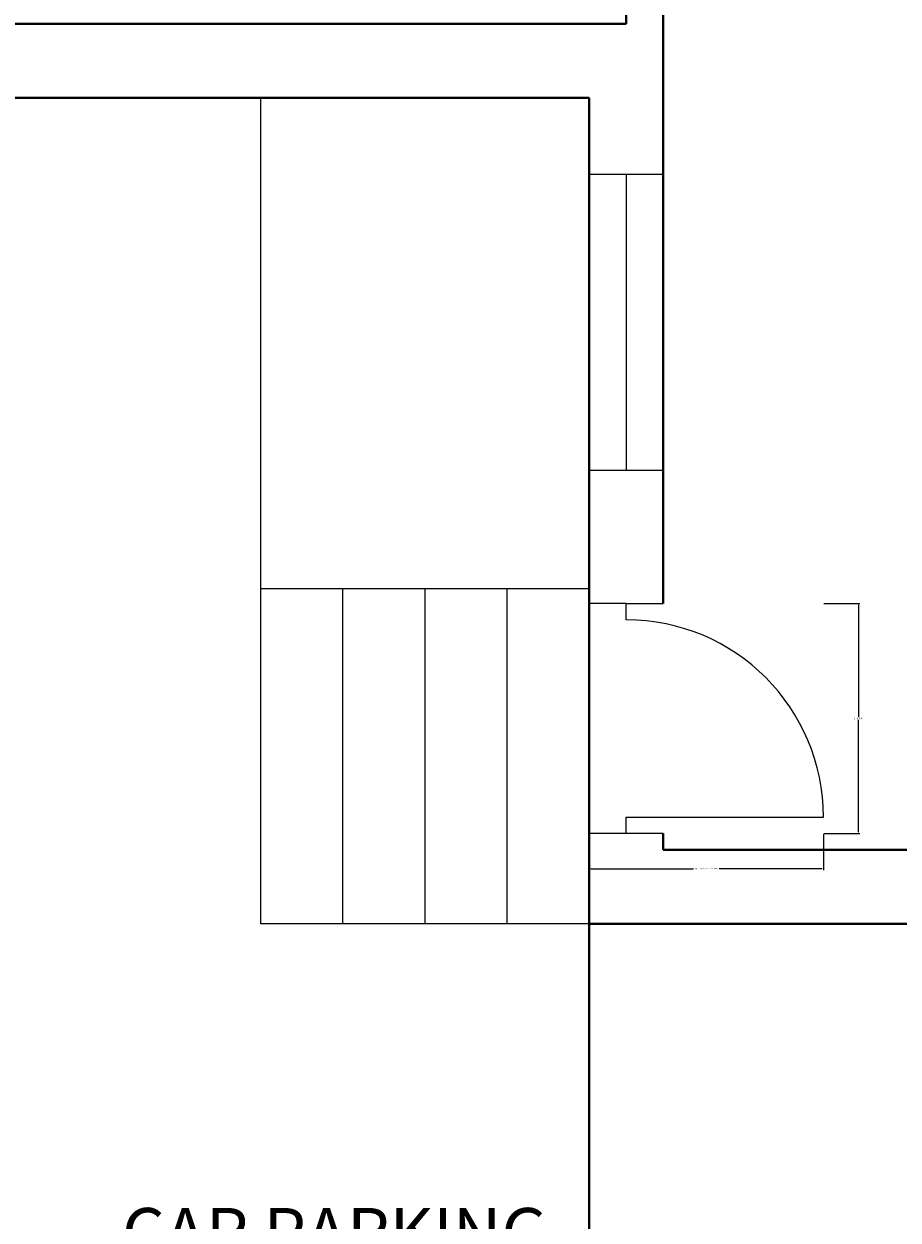
# Model space of a CAD drawing. Units: inches. Extents: x -19 to 419, y -828 to 43.
# Tile 4 of 9: x 126 to 233, y -720 to -574. Entities that reach past the tile are written whole.
import ezdxf

# ---------------------------------------------------------------- set-up
doc = ezdxf.new("R2010")
doc.units = ezdxf.units.IN
doc.header["$MEASUREMENT"] = 0
for name, color, linetype, lineweight in [('A-ANNO-DIMS', 2, 'Continuous', 18), ('A-AREA-IDEN', 7, 'Continuous', 25), ('A-DOOR', 3, 'Continuous', 25), ('A-FLOR-STRS', 7, 'Continuous', 25), ('A-GLAZ', 4, 'Continuous', 20), ('A-WALL', 7, 'Continuous', 40)]:
    doc.layers.add(name, color=color, linetype=linetype, lineweight=lineweight)
doc.styles.get("Standard").update_dxf_attribs({"font": 'arial.ttf'})
doc.dimstyles.get("Standard").update_dxf_attribs({"dimtxt": 0.18, "dimasz": 0.18, "dimexe": 0.18, "dimexo": 0.0625, "dimgap": 0.09, "dimtad": 0, "dimtih": 1, "dimtoh": 1, "dimdec": 0, "dimzin": 0, "dimdsep": 46, "dimlunit": 3, "dimtxsty": 'Standard', "dimcen": 0.09, "dimadec": 0, "dimazin": 0, "dimtfac": 1, "dimtdec": 0, "dimtofl": 0, "dimtmove": 0, "dimatfit": 3, "dimfxl": 1, "dimtolj": 1, "dimtzin": 0, "dimarcsym": 0})

# ---------------------------------------------------------------- blocks, each defined once
blk = doc.blocks.new('WIN-36X9')
for p, q in [((36, 9), (0, 9)), ((0, 9), (0, 0)), ((36, 0), (36, 9)), ((0, 4.5), (36, 4.5)), ((0, 0), (36, 0))]:
    blk.add_line(p, q)
blk = doc.blocks.new('DOOR-24-EXTERIOR')
for p, q in [((4.5, 28), (0, 28)), ((4.5, 26), (4.5, 28)), ((4.5, 28), (9, 28)), ((4.5, 0), (4.5, 2)), ((4.5, 2), (28.5, 2)), ((9, 0), (0, 0))]:
    blk.add_line(p, q)
blk.add_arc((4.5, 2), 24, 0, 90)
blk = doc.blocks.new('*D24')
at = {"layer": 'A-ANNO-DIMS', "color": 0, "lineweight": -2, "transparency": 16777216}
for p, q in [((195.24, -672.8), (195.24, -677.19)), ((223.74, -672.8), (223.74, -677.19)), ((195.42, -677.01), (207.92, -677.01)), ((223.56, -677.01), (211.06, -677.01))]:
    blk.add_line(p, q, dxfattribs=at)
at = {"layer": 'A-ANNO-DIMS', "color": 0, "transparency": 16777216}
for points in [[(195.42, -676.98), (195.42, -677.04), (195.24, -677.01)], [(223.56, -676.98), (223.56, -677.04), (223.74, -677.01)]]:
    blk.add_solid(points, dxfattribs=at)
at = {"layer": 'Defpoints', "color": 0, "transparency": 16777216}
for p in [(195.24, -672.73), (223.74, -672.73), (223.74, -677.01)]:
    blk.add_point(p, dxfattribs=at)
at = {"layer": 'A-ANNO-DIMS', "color": 0, "transparency": 16777216, "insert": (209.49, -677.01), "char_height": 0.18, "attachment_point": 5}
blk.add_mtext('\\A1;EXT. DOOR 2\'-4 1/2" TYP.', dxfattribs=at)
blk = doc.blocks.new('*D25')
at = {"layer": 'A-ANNO-DIMS', "color": 0, "lineweight": -2, "transparency": 16777216}
for p, q in [((223.8, -644.73), (228.19, -644.73)), ((228.01, -644.91), (228.01, -658.55)), ((228.01, -672.55), (228.01, -658.91)), ((223.8, -672.73), (228.19, -672.73))]:
    blk.add_line(p, q, dxfattribs=at)
at = {"layer": 'A-ANNO-DIMS', "color": 0, "transparency": 16777216}
for points in [[(227.98, -644.91), (228.04, -644.91), (228.01, -644.73)], [(227.98, -672.55), (228.04, -672.55), (228.01, -672.73)]]:
    blk.add_solid(points, dxfattribs=at)
at = {"layer": 'Defpoints', "color": 0, "transparency": 16777216}
for p in [(223.74, -644.73), (228.01, -644.73), (223.74, -672.73)]:
    blk.add_point(p, dxfattribs=at)
at = {"layer": 'A-ANNO-DIMS', "color": 0, "transparency": 16777216, "insert": (228.01, -658.73), "char_height": 0.18, "attachment_point": 5}
blk.add_mtext('\\A1;2\'-4" TYP.', dxfattribs=at)

msp = doc.modelspace()

# ---------------------------------------------------------------- linework, layer by layer
at = {"layer": 'A-FLOR-STRS'}
for p, q in [((155.24, -683.73), (155.24, -583.23)), ((195.24, -642.95), (155.24, -642.95)), ((165.24, -683.73), (165.24, -642.95)), ((175.24, -683.73), (175.24, -642.95)), ((185.24, -683.73), (185.24, -642.95)), ((165.24, -683.73), (155.24, -683.73)), ((175.24, -683.73), (165.24, -683.73)), ((185.24, -683.73), (175.24, -683.73)), ((195.24, -683.73), (185.24, -683.73))]:
    msp.add_line(p, q, dxfattribs=at)
at = {"layer": 'A-WALL'}
for p, q in [((199.74, -430.23), (199.74, -574.23)), ((204.24, -430.23), (204.24, -644.73)), ((31.74, -574.23), (199.74, -574.23)), ((22.74, -583.23), (195.24, -583.23)), ((195.24, -583.23), (195.24, -781.23)), ((204.24, -672.73), (204.24, -674.73)), ((204.24, -674.73), (400.74, -674.73)), ((195.24, -683.73), (400.74, -683.73))]:
    msp.add_line(p, q, dxfattribs=at)

# ---------------------------------------------------------------- block references
at = {"layer": 'A-DOOR'}
msp.add_blockref('DOOR-24-EXTERIOR', (195.24, -672.73), dxfattribs=at)
at = {"layer": 'A-GLAZ', "rotation": 269.9999999999998}
msp.add_blockref('WIN-36X9', (195.24, -592.54), dxfattribs=at)

# ---------------------------------------------------------------- texts
at = {"layer": 'A-AREA-IDEN', "insert": (138.35, -718.29), "char_height": 6, "attachment_point": 1}
msp.add_mtext('CAR PARKING\\P14\'0"X16\'6"', dxfattribs=at)

# ---------------------------------------------------------------- dimensions: what is measured, and where the dimension line sits
at = {"layer": 'A-ANNO-DIMS'}
dim = msp.add_linear_dim(base=(228.01, -644.73), p1=(223.74, -672.73), p2=(223.74, -644.73), angle=90, text='<> TYP.', dimstyle='Standard', override={"dimdec": 1, "dimlfac": 1, "dimrnd": 0, "dimzin": 1, "dimdsep": 46, "dimlunit": 4, "dimfrac": 2}, dxfattribs=at)
dim.commit()
dim.dimension.update_dxf_attribs({"geometry": '*D25', "text_midpoint": (228.01, -658.73)})
dim = msp.add_linear_dim(base=(223.74, -677.01), p1=(195.24, -672.73), p2=(223.74, -672.73), text='EXT. DOOR <> TYP.', dimstyle='Standard', override={"dimdec": 1, "dimlfac": 1, "dimrnd": 0, "dimzin": 1, "dimdsep": 46, "dimlunit": 4, "dimfrac": 2}, dxfattribs=at)
dim.commit()
dim.dimension.update_dxf_attribs({"geometry": '*D24', "text_midpoint": (209.49, -677.01)})

doc.saveas('drawing.dxf')
